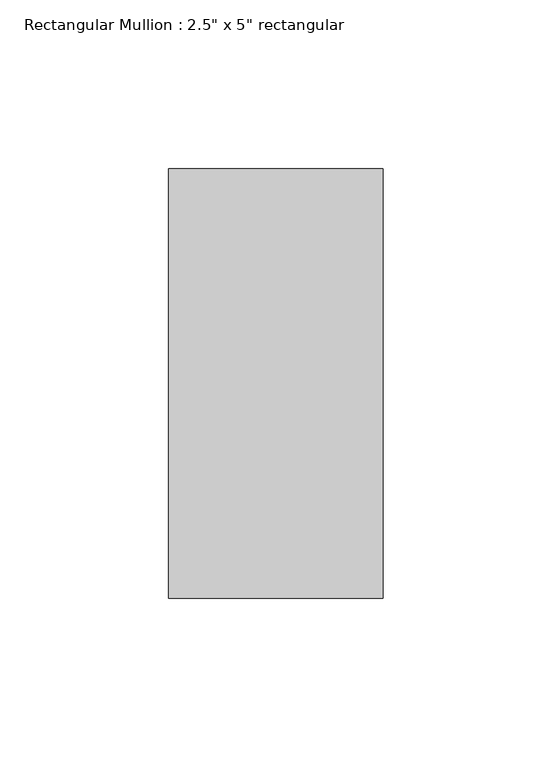
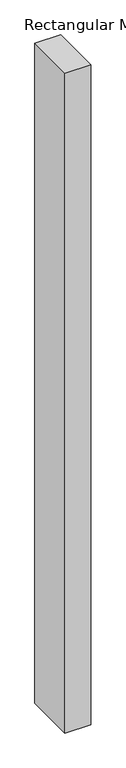
"""IFC4 building model written with IfcOpenShell, lengths in millimetres: member geometry."""

from ifc_helpers import new_model, si_unit, frame, origin, place, context, project, spatial, polyline, outline, extrude, source, transform, mapped, element, save


def member_4ab5fd4c(model_context):
    return source(origin(), model_context, "Body", "SweptSolid", [
        extrude(outline(polyline([(0.0, 63.5), (0.0, -63.5), (-63.5, -63.5), (-63.5, 63.5), (0.0, 63.5)])), frame((0.0, 0.0, -1708.8911809), z_axis=(0.0, 0.0, 1.0), x_axis=(1.0, 0.0, 0.0)), (0.0, 0.0, 1.0), 1708.8911809),
    ])


if __name__ == "__main__":
    model = new_model("IFC4")
    model_context = context("Model", 3, world=origin())
    ifc_project = project(units=[si_unit("LENGTHUNIT", "METRE", prefix="MILLI")], contexts=[model_context])
    site = spatial("IfcSite", under=ifc_project)
    building = spatial("IfcBuilding", under=site)
    placement = place(None, origin())
    member_shape = member_4ab5fd4c(model_context)
    element("IfcMember", 1, ObjectType="Rectangular Mullion : 2.5\" x 5\" rectangular", at=placement, inside=building, context=model_context, shape_type="MappedRepresentation", body=[
        mapped(member_shape, transform((0.0, 0.0, 0.0), x_axis=(1.0, 0.0, 0.0), y_axis=(0.0, 1.0, 0.0), z_axis=(0.0, 0.0, 1.0))),
    ])
    save(model, "model.ifc")

# Revit data of these elements
# Type "Rectangular Mullion : 2.5\" x 5\" rectangular"
#   built-in parameter 1007304 = 0.416667 (stored number, unit not read)
#   built-in parameter 1007301 = 0.104167 (stored number, unit not read)
#   built-in parameter 1007300 = 0.104167 (stored number, unit not read)
# Element 1 (IfcMember, "Rectangular Mullion : 2.5\" x 5\" rectangular")
#   Materials on its faces: "Aluminum"
# Materials
#   "Aluminum": class "Metal", colour RGB 247 247 247, transparency 0, Description = "Aluminum 6061", Cost = 0
